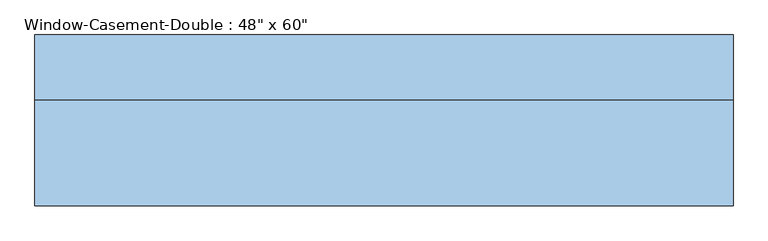
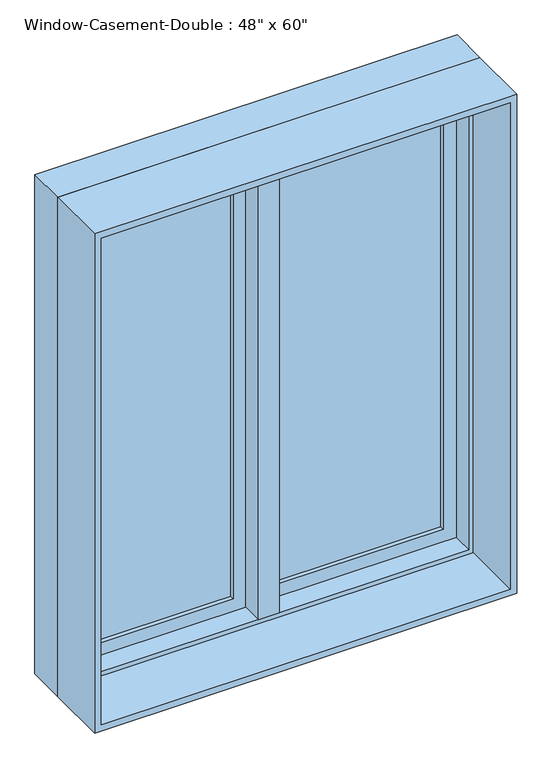
"""IFC4 building model written with IfcOpenShell, lengths in millimetres: window geometry."""

from ifc_helpers import new_model, si_unit, frame, origin, place, context, project, spatial, polyline, outline, extrude, faceted_brep, source, transform, mapped, element, save


def window_49c71971(model_context):
    return source(origin(), model_context, "Body", "SolidModel", [
        faceted_brep([(9.525, 158.75, 2425.7), (-9.525, 158.75, 2425.7), (-9.525, 107.95, 2425.7), (9.525, 107.95, 2425.7), (9.525, 158.75, 927.1), (9.525, 107.95, 927.1), (-9.525, 107.95, 927.1), (-9.525, 158.75, 927.1), (-9.525, 107.95, 946.15), (-9.525, 107.95, 2406.65), (-30.1625, 107.95, 946.15), (-30.1625, 107.95, 2406.65), (-30.1625, 44.45, 946.15), (-30.1625, 44.45, 2406.65), (30.1625, 44.45, 946.15), (30.1625, 44.45, 2406.65), (30.1625, 107.95, 946.15), (30.1625, 107.95, 2406.65), (9.525, 107.95, 946.15), (9.525, 107.95, 2406.65)], [[[0, 1, 2, 3]], [[4, 5, 6, 7]], [[1, 0, 4, 7]], [[2, 1, 7, 6, 8, 9]], [[9, 8, 10, 11]], [[11, 10, 12, 13]], [[13, 12, 14, 15]], [[15, 14, 16, 17]], [[17, 16, 18, 19]], [[0, 3, 19, 18, 5, 4]], [[18, 8, 6, 5]], [[9, 19, 3, 2]], [[8, 18, 16, 14, 12, 10]], [[19, 9, 11, 13, 15, 17]]]),
        extrude(outline(polyline([(-66.675, 139.7), (-66.675, 133.35), (-539.75, 133.35), (-539.75, 139.7), (-66.675, 139.7)])), frame((0.0, 0.0, 984.25), z_axis=(0.0, 0.0, 1.0), x_axis=(1.0, 0.0, 0.0)), (0.0, 0.0, 1.0), 1384.3),
        extrude(outline(polyline([(-539.75, 120.65), (-539.75, 127.0), (-66.675, 127.0), (-66.675, 120.65), (-539.75, 120.65)])), frame((0.0, 0.0, 984.25), z_axis=(0.0, 0.0, 1.0), x_axis=(1.0, 0.0, 0.0)), (0.0, 0.0, 1.0), 1384.3),
        extrude(outline(polyline([(539.75, 139.7), (539.75, 133.35), (66.675, 133.35), (66.675, 139.7), (539.75, 139.7)])), frame((0.0, 0.0, 984.25), z_axis=(0.0, 0.0, 1.0), x_axis=(1.0, 0.0, 0.0)), (0.0, 0.0, 1.0), 1384.3),
        extrude(outline(polyline([(66.675, 120.65), (66.675, 127.0), (539.75, 127.0), (539.75, 120.65), (66.675, 120.65)])), frame((0.0, 0.0, 984.25), z_axis=(0.0, 0.0, 1.0), x_axis=(1.0, 0.0, 0.0)), (0.0, 0.0, 1.0), 1384.3),
        extrude(outline(polyline([(2425.7, -596.9), (927.1, -596.9), (927.1, -9.525), (2425.7, -9.525), (2425.7, -596.9)]), holes=[polyline([(2368.55, -66.675), (984.25, -66.675), (984.25, -539.75), (2368.55, -539.75), (2368.55, -66.675)])]), frame((0.0, 107.95, 0.0), z_axis=(0.0, 1.0, 0.0), x_axis=(0.0, 0.0, 1.0)), (0.0, 0.0, 1.0), 44.45),
        extrude(outline(polyline([(927.1, 596.9), (2425.7, 596.9), (2425.7, 9.525), (927.1, 9.525), (927.1, 596.9)]), holes=[polyline([(984.25, 66.675), (2368.55, 66.675), (2368.55, 539.75), (984.25, 539.75), (984.25, 66.675)])]), frame((0.0, 107.95, 0.0), z_axis=(0.0, 1.0, 0.0), x_axis=(0.0, 0.0, 1.0)), (0.0, 0.0, 1.0), 44.45),
        extrude(outline(polyline([(2438.4, -609.6), (914.4, -609.6), (914.4, 609.6), (2438.4, 609.6), (2438.4, -609.6)]), holes=[polyline([(2419.35, 590.55), (933.45, 590.55), (933.45, -590.55), (2419.35, -590.55), (2419.35, 590.55)])]), frame((0.0, -139.7, 0.0), z_axis=(0.0, 1.0, 0.0), x_axis=(0.0, 0.0, 1.0)), (0.0, 0.0, 1.0), 184.15),
        faceted_brep([(577.85, 107.95, 2406.65), (577.85, 44.45, 2406.65), (-577.85, 44.45, 2406.65), (-577.85, 107.95, 2406.65), (596.9, 158.75, 2425.7), (596.9, 107.95, 2425.7), (-596.9, 107.95, 2425.7), (-596.9, 158.75, 2425.7), (609.6, 44.45, 2438.4), (609.6, 158.75, 2438.4), (-609.6, 158.75, 2438.4), (-609.6, 44.45, 2438.4), (-577.85, 44.45, 946.15), (-577.85, 107.95, 946.15), (-596.9, 107.95, 927.1), (-596.9, 158.75, 927.1), (-609.6, 158.75, 914.4), (-609.6, 44.45, 914.4), (577.85, 44.45, 946.15), (577.85, 107.95, 946.15), (596.9, 107.95, 927.1), (596.9, 158.75, 927.1), (609.6, 158.75, 914.4), (609.6, 44.45, 914.4)], [[[0, 1, 2, 3]], [[4, 5, 6, 7]], [[8, 9, 10, 11]], [[3, 2, 12, 13]], [[7, 6, 14, 15]], [[11, 10, 16, 17]], [[13, 12, 18, 19]], [[15, 14, 20, 21]], [[17, 16, 22, 23]], [[11, 17, 23, 8], [1, 18, 12, 2]], [[19, 18, 1, 0]], [[5, 20, 14, 6], [3, 13, 19, 0]], [[21, 20, 5, 4]], [[23, 22, 9, 8]], [[9, 22, 16, 10], [7, 15, 21, 4]]]),
    ])


if __name__ == "__main__":
    model = new_model("IFC4")
    model_context = context("Model", 3, world=origin())
    ifc_project = project(units=[si_unit("LENGTHUNIT", "METRE", prefix="MILLI")], contexts=[model_context])
    site = spatial("IfcSite", under=ifc_project)
    building = spatial("IfcBuilding", under=site)
    placement = place(None, origin())
    window_shape = window_49c71971(model_context)
    element("IfcWindow", 1, ObjectType="Window-Casement-Double : 48\" x 60\"", at=placement, inside=building, context=model_context, shape_type="MappedRepresentation", body=[
        mapped(window_shape, transform((0.0, 0.0, 0.0), x_axis=(1.0, 0.0, 0.0), y_axis=(0.0, 1.0, 0.0), z_axis=(0.0, 0.0, 1.0))),
    ])
    save(model, "model.ifc")

# Revit data of these elements
# Type "Window-Casement-Double : 48\" x 60\""
#   Type Mark = "16"
#   Fire Rating = "0.5h"
#   Assembly Code = "B2020100"
#   Analytic Construction = "Double glazing - domestic"
#   Frame Extension [instance default] = 0' - 0 1/4"
#   Window Inset [instance default] = 0' - 0"
#   Wall Thickness [instance default] = 0' - 6"
#   Interior Wall Closure [instance default] = 0' - 2 1/4"
#   Half Width = 2' - 0"
#   Visual Light Transmittance = 0.81
#   Thermal Resistance (R) = 1.8146 (h·ft²·°F)/BTU
#   Solar Heat Gain Coefficient = 0.76
#   Rough Width = 4' - 0 1/2"
#   Rough Height = 5' - 0 1/2"
#   Height = 5' - 0"
#   Heat Transfer Coefficient (U) = 0.5511 BTU/(h·ft²·°F)
#   Exterior Wall Closure [instance default] = 0' - 1 1/4"
#   Extension Jamb [instance default] = 0' - 2 1/4"
#   Default Sill Height = 3' - 0"
#   Width = 4' - 0"
#   Define Thermal Properties by = 0
#   Muntin Visibility = yes
#   Interior Trim Visibility [instance default] = yes
#   Exterior Trim Visibility [instance default] = yes
#   Extension Jamb Visibility [instance default] = yes
#   Interior Trim Material = Wood - Stained
#   Muntin Pattern = Muntin Pattern_2x2 : Muntin Pattern_2x2
#   Interior Trim = Trim-Window-Interior-Flat : Picture Frame
#   Interior Frame Material = Wood - Stained
#   Glass Panel Material = Glass
#   Exterior Trim Material = Clad - White
#   Exterior Trim = Trim-Window-Exterior-Flat : with Sill
#   Exterior Frame Material = Clad - White
#   Wall Closure = (empty or 0)
# Element 1 (IfcWindow, "Window-Casement-Double : 48\" x 60\"")
#   Wall Thickness = 0' - 11"
#   Extension Jamb = 0' - 7 1/4"
#   Materials on its faces: "Wood - Stained", "Glass", "Clad - White"
# Materials
#   "Wood - Stained": class "Wood", colour RGB 224 178 126, transparency 0, Cost = 0
#   "Glass": class "Glass", colour RGB 0 128 192, transparency 0.75, Description = "Soda Lime Glass", Cost = 0
#   "Clad - White": class "Wood", colour RGB 242 242 238, transparency 0, Cost = 0
